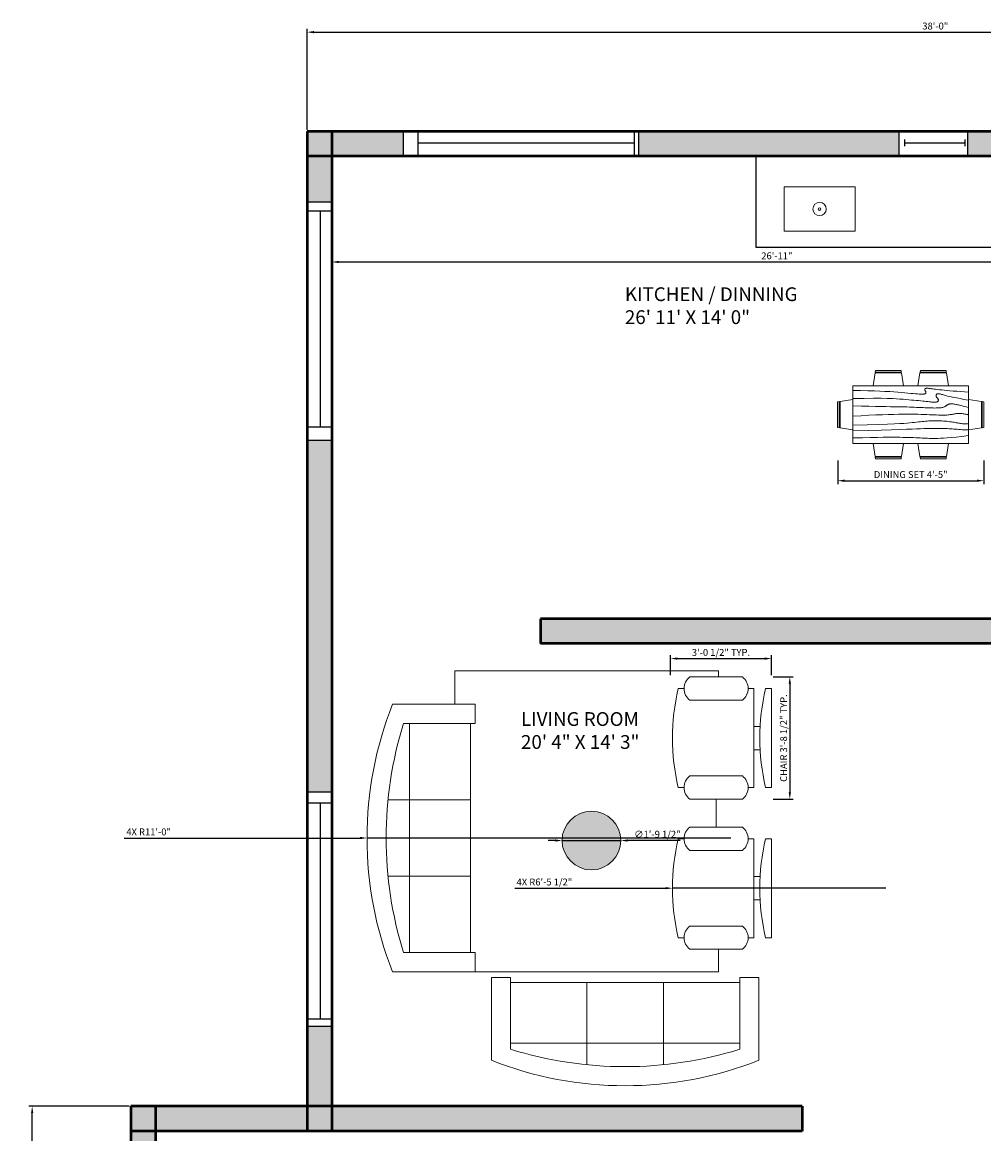
# Model space of a CAD drawing. Units: millimetres. Extents: x 2481 to 3088, y 720 to 1513.
# Tile 3 of 4: x 2487 to 2836, y 1109 to 1513. Entities that reach past the tile are written whole.
import ezdxf

# ---------------------------------------------------------------- set-up
doc = ezdxf.new("R2010")
doc.units = ezdxf.units.MM
for name, color, linetype, lineweight in [('A-FLOR-CASE', 150, 'Continuous', 25), ('A-FLOR-FIXT', 2, 'Continuous', 18), ('A-FURN-PATT', 3, 'Continuous', 13), ('A-WALL-PATT', 5, 'Continuous', 13), ('DIMENSIONS', 10, 'Continuous', 18), ('FURNITURE', 2, 'Continuous', 18), ('TEXT', 80, 'Continuous', 25), ('WALLS', 150, 'Continuous', 50), ('WINDOWS', 23, 'Continuous', 25)]:
    doc.layers.add(name, color=color, linetype=linetype, lineweight=lineweight)
doc.styles.get("Standard").update_dxf_attribs({"font": 'arial.ttf'})
doc.dimstyles.new('ISO-25', dxfattribs={"dimtxt": 2.5, "dimasz": 2.5, "dimexe": 1.25, "dimexo": 0.625, "dimtad": 1, "dimdec": 0, "dimlunit": 3, "dimtxsty": 'Standard', "dimcen": 2.5, "dimadec": 0, "dimazin": 0, "dimtfac": 1, "dimtdec": 0, "dimtmove": 0, "dimatfit": 3, "dimfxl": 1, "dimarcsym": 0})

# ---------------------------------------------------------------- blocks, each defined once
blk = doc.blocks.new('*U4')
for p, q in [((0, 4), (0, 0)), ((36, 4), (36, 0)), ((0, 2), (36, 2))]:
    blk.add_line(p, q)
blk = doc.blocks.new('*U6')
for p, q in [((0, 4), (0, 0)), ((0, 2), (36, 2)), ((36, 4), (36, 0))]:
    blk.add_line(p, q)
blk = doc.blocks.new('Dining Set - 36 x 72 in.')
for p, q in [((-22.2343, 26.00059), (-23.4847, 17.99762)), ((-22.2304, 26), (-5.7608, 26)), ((-22, 27.5), (-22.1562, 26.50042)), ((-5.8416, 26.5), (-22.1534, 26.5)), ((-22, 27.5), (-6, 27.5)), ((-5.8437, 26.49966), (-6, 27.5)), ((-4.5152, 17.99762), (-5.7655, 25.99926)), ((5.7657, 26.00059), (4.5153, 17.99762)), ((5.7696, 26), (22.2392, 26)), ((6, 27.5), (5.8438, 26.50042)), ((22.1584, 26.5), (5.8466, 26.5)), ((6, 27.5), (22, 27.5)), ((22.1563, 26.49966), (22, 27.5)), ((23.4848, 17.99762), (22.2345, 25.99926)), ((36, 18), (-36, 18)), ((-36, 18), (-36, -18)), ((36, -18), (36, 18)), ((-45.5, 8), (-44.5004, 8.15617)), ((-45.5, 8), (-45.5, -8)), ((-44.5, -8.15843), (-44.5, 8.15338)), ((-44.0006, 8.23428), (-35.9976, 9.48474)), ((-44, 8.23041), (-44, -8.23915)), ((44.0006, 8.23428), (35.9976, 9.48474)), ((44, 8.23041), (44, -8.23915)), ((44.5, -8.15843), (44.5, 8.15338)), ((45.5, 8), (44.5005, 8.15617)), ((45.5, 8), (45.5, -8)), ((-44.4997, -8.15631), (-45.5, -8)), ((-35.9976, -9.48476), (-43.9993, -8.2345)), ((35.9976, -9.48476), (43.9993, -8.2345)), ((44.4997, -8.15631), (45.5, -8)), ((-36, -18), (36, -18)), ((-22.2343, -26.0006), (-23.4847, -17.99762)), ((-4.5152, -17.99762), (-5.7655, -25.99928)), ((5.7657, -26.0006), (4.5153, -17.99762)), ((23.4848, -17.99762), (22.2345, -25.99928)), ((-22.2304, -26), (-5.7608, -26)), ((-22, -27.5), (-22.1562, -26.50044)), ((-5.8416, -26.5), (-22.1534, -26.5)), ((-22, -27.5), (-6, -27.5)), ((-5.8437, -26.49967), (-6, -27.5)), ((5.7696, -26), (22.2392, -26)), ((6, -27.5), (5.8438, -26.50044)), ((22.1584, -26.5), (5.8466, -26.5)), ((6, -27.5), (22, -27.5)), ((22.1563, -26.49967), (22, -27.5))]:
    blk.add_line(p, q)
for points in [[(-36, 15), (-31.1772, 14.97754), (-26.8079, 14.91406), (-22.8538, 14.81543), (-19.276, 14.6875), (-16.0362, 14.53613), (-13.0957, 14.36718), (-10.4159, 14.18652), (-7.9583, 14), (-5.6904, 13.81315), (-3.6035, 13.63021), (-1.6954, 13.45508), (0.0365, 13.29166), (1.5945, 13.14388), (2.9811, 13.01562), (4.1988, 12.9108), (5.25, 12.83333), (6.1393, 12.78613), (6.8802, 12.76823), (7.4883, 12.77767), (7.9792, 12.8125), (8.3685, 12.87077), (8.6719, 12.95052), (8.9049, 13.0498), (9.0833, 13.16666), (9.2205, 13.29899), (9.3216, 13.44401), (9.3895, 13.59879), (9.4271, 13.76041), (9.4373, 13.92594), (9.4232, 14.09245), (9.3875, 14.257), (9.3333, 14.41666), (9.2638, 14.56917), (9.1836, 14.71484), (9.0975, 14.85465), (9.0104, 14.98958), (8.9272, 15.1206), (8.8529, 15.2487), (8.7922, 15.37483), (8.75, 15.5), (8.7305, 15.62467), (8.7344, 15.74739), (8.7617, 15.86621), (8.8125, 15.97916), (8.8867, 16.08431), (8.9844, 16.17968), (9.1055, 16.26334), (9.25, 16.33333), (9.4189, 16.38802), (9.6172, 16.42708), (9.8506, 16.45052), (10.125, 16.45833), (10.4463, 16.45052), (10.8203, 16.42708), (11.2529, 16.38802), (11.75, 16.33333), (12.3184, 16.26318), (12.9694, 16.17838), (13.7151, 16.07991), (14.5677, 15.96875), (15.5395, 15.84586), (16.6426, 15.71224), (17.8893, 15.56884), (19.2917, 15.41666), (20.859, 15.25667), (22.5879, 15.08984), (24.4721, 14.91715), (26.5052, 14.73958), (28.6809, 14.5581), (30.9929, 14.3737), (33.4347, 14.18733), (36, 14)], [(-36, 10), (-28.9766, 10.14274), (-23.1725, 10.20442), (-18.4241, 10.19775), (-14.5677, 10.13541), (-11.4399, 10.03011), (-8.877, 9.89453), (-6.7154, 9.74137), (-4.7917, 9.58333), (-2.9698, 9.43082), (-1.2246, 9.28515), (0.4415, 9.14534), (2.026, 9.01041), (3.5266, 8.87939), (4.9408, 8.7513), (6.266, 8.62516), (7.5, 8.5), (8.6411, 8.37549), (9.6914, 8.2539), (10.6538, 8.13818), (11.5312, 8.03125), (12.3267, 7.93603), (13.043, 7.85547), (13.6831, 7.79248), (14.25, 7.75), (14.7471, 7.7303), (15.1797, 7.73307), (15.5537, 7.75732), (15.875, 7.80208), (16.1494, 7.86637), (16.3828, 7.94922), (16.5811, 8.04964), (16.75, 8.16666), (16.8944, 8.29915), (17.0143, 8.44531), (17.1089, 8.60319), (17.1771, 8.77083), (17.218, 8.94629), (17.2305, 9.1276), (17.2137, 9.31282), (17.1667, 9.5), (17.0895, 9.6875), (16.987, 9.875), (16.8649, 10.0625), (16.7292, 10.25), (16.5856, 10.4375), (16.4401, 10.625), (16.2985, 10.8125), (16.1667, 11), (16.05, 11.18733), (15.9518, 11.3737), (15.8752, 11.5581), (15.8229, 11.73958), (15.798, 11.91715), (15.8034, 12.08984), (15.842, 12.25667), (15.9167, 12.41666), (16.0295, 12.56836), (16.1784, 12.70833), (16.3605, 12.83268), (16.5729, 12.9375), (16.8127, 13.01888), (17.0768, 13.07291), (17.3625, 13.0957), (17.6667, 13.08333), (17.9894, 13.03312), (18.3418, 12.94726), (18.7382, 12.82918), (19.1927, 12.68229), (19.7195, 12.51001), (20.3327, 12.31575), (21.0465, 12.10294), (21.875, 11.875), (22.8357, 11.63354), (23.959, 11.37304), (25.2786, 11.08618), (26.8282, 10.76562), (28.6414, 10.40405), (30.752, 9.99414), (33.1936, 9.52856), (36, 9)], [(-36, 5.5), (-30.7157, 5.3348), (-26.069, 5.20963), (-21.9946, 5.11767), (-18.4271, 5.05208), (-15.3009, 5.00602), (-12.5508, 4.97265), (-10.1112, 4.94515), (-7.9167, 4.91666), (-5.909, 4.88167), (-4.0586, 4.83984), (-2.3429, 4.79215), (-0.7396, 4.73958), (0.7739, 4.6831), (2.22, 4.6237), (3.6213, 4.56233), (5, 4.5), (6.373, 4.43782), (7.7344, 4.3776), (9.0723, 4.32129), (10.375, 4.27083), (11.6309, 4.22819), (12.8281, 4.19531), (13.9551, 4.17415), (15, 4.16666), (15.954, 4.17448), (16.819, 4.19791), (17.6001, 4.23698), (18.3021, 4.29166), (18.9299, 4.36198), (19.4883, 4.44791), (19.9823, 4.54948), (20.4167, 4.66666), (20.7969, 4.79899), (21.1302, 4.94401), (21.4245, 5.09879), (21.6875, 5.26041), (21.9271, 5.42594), (22.1511, 5.59245), (22.3672, 5.757), (22.5834, 5.91666), (22.8065, 6.06868), (23.0404, 6.21093), (23.2879, 6.34147), (23.5521, 6.45833), (23.8358, 6.55957), (24.142, 6.64323), (24.4735, 6.70735), (24.8334, 6.75), (25.2235, 6.76969), (25.642, 6.76692), (26.0858, 6.74267), (26.5521, 6.69791), (27.0379, 6.63362), (27.5404, 6.55078), (28.0565, 6.45036), (28.5834, 6.33333), (29.1242, 6.19987), (29.7071, 6.04687), (30.3661, 5.87044), (31.1354, 5.66666), (32.0493, 5.43164), (33.142, 5.16146), (34.4475, 4.85221), (36, 4.5)], [(-36, -1), (-30.7915, -0.6591), (-26.0195, -0.38216), (-21.6519, -0.16284), (-17.6563, 0.00521), (-14.0005, 0.12833), (-10.6523, 0.21289), (-7.5796, 0.26522), (-4.75, 0.29166), (-2.134, 0.29793), (0.2878, 0.28711), (2.5317, 0.26163), (4.6146, 0.22396), (6.5529, 0.17651), (8.3633, 0.12174), (10.0623, 0.06209), (11.6667, 0), (13.1899, -0.06201), (14.6341, -0.1211), (15.9982, -0.17432), (17.2813, -0.21875), (18.4823, -0.25147), (19.6003, -0.26953), (20.6343, -0.27002), (21.5834, -0.25), (22.4481, -0.20768), (23.2357, -0.14584), (23.9549, -0.06836), (24.6146, 0.02083), (25.2235, 0.11784), (25.7904, 0.21875), (26.3241, 0.31966), (26.8334, 0.41666), (27.3265, 0.50618), (27.8099, 0.58593), (28.2894, 0.65397), (28.7709, 0.70833), (29.2601, 0.74707), (29.763, 0.76823), (30.2855, 0.76985), (30.8334, 0.75), (31.4088, 0.70784), (31.9994, 0.64713), (32.589, 0.57275), (33.1615, 0.48958), (33.7008, 0.4025), (34.1908, 0.3164), (34.6153, 0.23616), (34.9584, 0.16666), (35.2099, 0.11165), (35.3848, 0.07031), (35.504, 0.04069), (35.5886, 0.02083), (35.6594, 0.00879), (35.7377, 0.0026), (35.8442, 0.00032), (36, 0)], [(-36, -6.5), (-27.1843, -6.31267), (-20.084, -6.1263), (-14.469, -5.9419), (-10.1094, -5.76042), (-6.7752, -5.58285), (-4.2363, -5.41016), (-2.2629, -5.24333), (-0.625, -5.08334), (0.8708, -4.93099), (2.2715, -4.78646), (3.5872, -4.64974), (4.8281, -4.52084), (6.0046, -4.39974), (7.127, -4.28646), (8.2053, -4.18099), (9.25, -4.08334), (10.2705, -3.99382), (11.2734, -3.91407), (12.2647, -3.84603), (13.25, -3.79167), (14.2354, -3.75293), (15.2266, -3.73177), (16.2295, -3.73015), (17.25, -3.75), (18.2912, -3.79248), (19.3451, -3.85547), (20.4009, -3.93604), (21.4479, -4.03125), (22.4754, -4.13819), (23.4727, -4.25391), (24.4289, -4.37549), (25.3334, -4.5), (26.1785, -4.62492), (26.9694, -4.74935), (27.7145, -4.87281), (28.4219, -4.99479), (29.1, -5.11483), (29.7572, -5.23242), (30.4016, -5.34709), (31.0417, -5.45834), (31.6837, -5.56437), (32.3262, -5.65821), (32.9658, -5.73153), (33.599, -5.77604), (34.2224, -5.78345), (34.8327, -5.74545), (35.4264, -5.65373), (36, -5.5)], [(-36, -10), (-26.4022, -9.81299), (-18.4675, -9.62891), (-11.9839, -9.45069), (-6.7396, -9.28125), (-2.5226, -9.12354), (0.8789, -8.98047), (3.6769, -8.85498), (6.0833, -8.75), (8.2767, -8.66765), (10.3021, -8.60677), (12.1712, -8.56543), (13.8958, -8.54167), (15.4876, -8.53353), (16.9583, -8.53907), (18.3197, -8.55632), (19.5834, -8.58334), (20.7616, -8.61841), (21.8685, -8.66081), (22.9188, -8.71004), (23.9271, -8.76563), (24.9081, -8.82707), (25.8763, -8.89388), (26.8465, -8.96558), (27.8334, -9.04167), (28.8474, -9.12118), (29.8828, -9.20117), (30.93, -9.27824), (31.9792, -9.34896), (33.0205, -9.40991), (34.0443, -9.45768), (35.0407, -9.48885), (36, -9.5)], [(-36, -14.5), (-30.0881, -14.33513), (-25.0332, -14.21224), (-20.7312, -14.12647), (-17.0781, -14.07292), (-13.97, -14.04671), (-11.3027, -14.04297), (-8.9724, -14.05681), (-6.875, -14.08334), (-4.9224, -14.11833), (-3.0905, -14.16016), (-1.3709, -14.20785), (0.2448, -14.26042), (1.7647, -14.3169), (3.1973, -14.3763), (4.5507, -14.43767), (5.8333, -14.5), (7.0554, -14.5621), (8.235, -14.62175), (9.3922, -14.67652), (10.5469, -14.72396), (11.7192, -14.76164), (12.929, -14.78711), (14.1965, -14.79794), (15.5417, -14.79167), (16.9933, -14.76424), (18.6152, -14.70508), (20.4804, -14.60197), (22.6615, -14.44271), (25.2312, -14.21509), (28.2624, -13.9069), (31.8277, -13.50594), (36, -13)]]:
    blk.add_lwpolyline(points)
blk = doc.blocks.new('Sofa - Roundback 7 ft.')
for p, q in [((-12.00002, -32.4421), (-12.00003, -6.5971)), ((11.99997, -32.4421), (11.99998, -6.5971)), ((-36.000027, -34), (-36.000027, -11.4696)), ((-35.999844, -13.3819), (35.9998, -13.3819)), ((35.99998, -34), (35.99998, -11.4696)), ((-36.000027, -32.4421), (35.99998, -32.4421))]:
    blk.add_line(p, q)
for points in [[(-36.000027, -34), (-42.000027, -34), (-42.000027, -8)], [(41.99998, -8), (41.99998, -34), (35.99998, -34)]]:
    blk.add_lwpolyline(points)
for centre, radius, start, end in [((0, -114.25), 114.25, 68.43141, 111.5686), ((-0.00001, -127.1968), 121.1968, 72.72033, 107.2797)]:
    blk.add_arc(centre, radius, start, end)
blk = doc.blocks.new('Chair - Desk')
for p, q in [((-8.5, 0), (-8.5, -1)), ((-8.5, 0), (8.5, 0)), ((8.5, 0), (8.5, -1)), ((-8.5, -3), (-8.5, -4)), ((-8.5, -3), (8.5, -3)), ((-2, -3), (-2, -1.9355)), ((2, -1.9576), (2, -3)), ((8.5, -3), (8.5, -4)), ((-10.5, -5), (-10.5, -14)), ((-6.5, -14), (-6.5, -5)), ((6.5, -5), (6.5, -14)), ((10.5, -14), (10.5, -5)), ((-8.5, -15), (-8.5, -16)), ((8.5, -15), (8.5, -16))]:
    blk.add_line(p, q)
for centre, radius, start, end in [((0, 34.625), 36.625, 256.5803, 283.4197), ((-8.5, -6.5), 2.5, 36.8699, 143.1301), ((8.5, -6.5), 2.5, 36.8699, 143.1301), ((-8.5, -12.5), 2.5, 216.8699, 323.1301), ((8.5, -12.5), 2.5, 216.8699, 323.1301), ((0, 19.625), 36.625, 256.5803, 283.4197)]:
    blk.add_arc(centre, radius, start, end)
blk = doc.blocks.new('*D16')
at = {"layer": 'Defpoints', "color": 0, "transparency": 16777216}
for p in [(2599.5, 1428.42), (2922.5, 1426.09), (2922.5, 1426.09)]:
    blk.add_point(p, dxfattribs=at)
at = {"layer": 'DIMENSIONS', "color": 0, "lineweight": -2, "transparency": 16777216}
for p, q in [((2599.5, 1427.79), (2599.5, 1424.84)), ((2602, 1426.09), (2920, 1426.09)), ((2922.5, 1426.72), (2922.5, 1427.34))]:
    blk.add_line(p, q, dxfattribs=at)
at = {"layer": 'DIMENSIONS', "color": 0, "transparency": 16777216}
for points in [[(2602, 1426.51), (2602, 1425.68), (2599.5, 1426.09)], [(2920, 1426.51), (2920, 1425.68), (2922.5, 1426.09)]]:
    blk.add_solid(points, dxfattribs=at)
at = {"layer": 'DIMENSIONS', "color": 0, "transparency": 16777216, "insert": (2761, 1428), "char_height": 2.5, "attachment_point": 5}
blk.add_mtext('26\'-11"', dxfattribs=at)
blk = doc.blocks.new('*D29')
at = {"layer": 'Defpoints', "color": 0, "transparency": 16777216}
for p in [(2759.04, 1275.4), (2759.04, 1230.99), (2765.7, 1230.99)]:
    blk.add_point(p, dxfattribs=at)
at = {"layer": 'DIMENSIONS', "color": 0, "lineweight": -2, "transparency": 16777216}
for p, q in [((2759.66, 1275.4), (2766.95, 1275.4)), ((2765.7, 1272.9), (2765.7, 1233.49)), ((2759.66, 1230.99), (2766.95, 1230.99))]:
    blk.add_line(p, q, dxfattribs=at)
at = {"layer": 'DIMENSIONS', "color": 0, "transparency": 16777216}
for points in [[(2765.28, 1272.9), (2766.11, 1272.9), (2765.7, 1275.4)], [(2765.28, 1233.49), (2766.11, 1233.49), (2765.7, 1230.99)]]:
    blk.add_solid(points, dxfattribs=at)
at = {"layer": 'DIMENSIONS', "color": 0, "transparency": 16777216, "insert": (2763.78, 1253.19), "char_height": 2.5, "attachment_point": 5, "rotation": 90}
blk.add_mtext('CHAIR 3\'-8 1/2" TYP.', dxfattribs=at)
blk = doc.blocks.new('*D30')
at = {"layer": 'Defpoints', "color": 0, "transparency": 16777216}
for p in [(2759.04, 1282.06), (2722.39, 1275.4), (2759.04, 1275.4)]:
    blk.add_point(p, dxfattribs=at)
at = {"layer": 'DIMENSIONS', "color": 0, "lineweight": -2, "transparency": 16777216}
for p, q in [((2722.39, 1276.02), (2722.39, 1283.31)), ((2724.89, 1282.06), (2756.54, 1282.06)), ((2759.04, 1276.02), (2759.04, 1283.31))]:
    blk.add_line(p, q, dxfattribs=at)
at = {"layer": 'DIMENSIONS', "color": 0, "transparency": 16777216}
for points in [[(2724.89, 1282.47), (2724.89, 1281.64), (2722.39, 1282.06)], [(2756.54, 1282.47), (2756.54, 1281.64), (2759.04, 1282.06)]]:
    blk.add_solid(points, dxfattribs=at)
at = {"layer": 'DIMENSIONS', "color": 0, "transparency": 16777216, "insert": (2740.71, 1283.97), "char_height": 2.5, "attachment_point": 5}
blk.add_mtext('3\'-0 1/2" TYP.', dxfattribs=at)
blk = doc.blocks.new('*D33')
at = {"layer": 'Defpoints', "color": 0, "transparency": 16777216}
for p in [(2783.07, 1354.61), (2836.1, 1354.61), (2836.1, 1346.66)]:
    blk.add_point(p, dxfattribs=at)
at = {"layer": 'DIMENSIONS', "color": 0, "lineweight": -2, "transparency": 16777216}
for p, q in [((2783.07, 1353.98), (2783.07, 1345.41)), ((2836.1, 1353.98), (2836.1, 1345.41)), ((2785.57, 1346.66), (2833.6, 1346.66))]:
    blk.add_line(p, q, dxfattribs=at)
at = {"layer": 'DIMENSIONS', "color": 0, "transparency": 16777216}
for points in [[(2785.57, 1347.07), (2785.57, 1346.24), (2783.07, 1346.66)], [(2833.6, 1347.07), (2833.6, 1346.24), (2836.1, 1346.66)]]:
    blk.add_solid(points, dxfattribs=at)
at = {"layer": 'DIMENSIONS', "color": 0, "transparency": 16777216, "insert": (2809.58, 1348.57), "char_height": 2.5, "attachment_point": 5}
blk.add_mtext('DINING SET 4\'-5"', dxfattribs=at)
blk = doc.blocks.new('*D39')
at = {"layer": 'Defpoints', "color": 0, "transparency": 16777216}
for p in [(3046.5, 1509.55), (2590.5, 1473.49), (3046.5, 1473.49)]:
    blk.add_point(p, dxfattribs=at)
at = {"layer": 'DIMENSIONS', "color": 0, "lineweight": -2, "transparency": 16777216}
for p, q in [((2590.5, 1474.11), (2590.5, 1510.8)), ((3046.5, 1474.11), (3046.5, 1510.8)), ((2593, 1509.55), (3044, 1509.55))]:
    blk.add_line(p, q, dxfattribs=at)
at = {"layer": 'DIMENSIONS', "color": 0, "transparency": 16777216}
for points in [[(2593, 1509.97), (2593, 1509.13), (2590.5, 1509.55)], [(3044, 1509.97), (3044, 1509.13), (3046.5, 1509.55)]]:
    blk.add_solid(points, dxfattribs=at)
at = {"layer": 'DIMENSIONS', "color": 0, "transparency": 16777216, "insert": (2818.5, 1511.45), "char_height": 2.5, "attachment_point": 5}
blk.add_mtext('38\'-0"', dxfattribs=at)
blk = doc.blocks.new('*D40')
at = {"layer": 'Defpoints', "color": 0, "transparency": 16777216}
for p in [(2490.69, 1119.49), (2526.5, 1119.49), (2526.5, 765.49)]:
    blk.add_point(p, dxfattribs=at)
at = {"layer": 'DIMENSIONS', "color": 0, "lineweight": -2, "transparency": 16777216}
for p, q in [((2525.87, 1119.49), (2489.44, 1119.49)), ((2490.69, 767.99), (2490.69, 1116.99)), ((2525.87, 765.49), (2489.44, 765.49))]:
    blk.add_line(p, q, dxfattribs=at)
at = {"layer": 'DIMENSIONS', "color": 0, "transparency": 16777216}
for points in [[(2490.28, 1116.99), (2491.11, 1116.99), (2490.69, 1119.49)], [(2490.28, 767.99), (2491.11, 767.99), (2490.69, 765.49)]]:
    blk.add_solid(points, dxfattribs=at)
at = {"layer": 'DIMENSIONS', "color": 0, "transparency": 16777216, "insert": (2488.79, 942.49), "char_height": 2.5, "attachment_point": 5, "rotation": 90}
blk.add_mtext('29\'-6"', dxfattribs=at)
blk = doc.blocks.new('*D48')
at = {"layer": 'Defpoints', "color": 0, "transparency": 16777216}
for p in [(2612.23, 1216.89), (2744.32, 1216.89)]:
    blk.add_point(p, dxfattribs=at)
at = {"layer": 'DIMENSIONS', "color": 0, "lineweight": -2, "transparency": 16777216}
for p, q in [((2524.12, 1216.89), (2609.73, 1216.89)), ((2744.32, 1216.89), (2612.23, 1216.89))]:
    blk.add_line(p, q, dxfattribs=at)
at = {"layer": 'DIMENSIONS', "color": 0, "transparency": 16777216}
blk.add_solid([(2609.73, 1217.31), (2609.73, 1216.48), (2612.23, 1216.89)], dxfattribs=at)
at = {"layer": 'DIMENSIONS', "color": 0, "transparency": 16777216, "insert": (2532.97, 1218.79), "char_height": 2.5, "attachment_point": 5, "rotation": 359.9998}
blk.add_mtext('4X R11\'-0"', dxfattribs=at)
blk = doc.blocks.new('*D49')
at = {"layer": 'Defpoints', "color": 0, "transparency": 16777216}
for p in [(2723.09, 1198.67), (2800.53, 1198.67)]:
    blk.add_point(p, dxfattribs=at)
at = {"layer": 'DIMENSIONS', "color": 0, "lineweight": -2, "transparency": 16777216}
for p, q in [((2665.84, 1198.67), (2720.59, 1198.67)), ((2800.53, 1198.67), (2723.09, 1198.67))]:
    blk.add_line(p, q, dxfattribs=at)
at = {"layer": 'DIMENSIONS', "color": 0, "transparency": 16777216}
blk.add_solid([(2720.59, 1199.09), (2720.59, 1198.26), (2723.09, 1198.67)], dxfattribs=at)
at = {"layer": 'DIMENSIONS', "color": 0, "transparency": 16777216, "insert": (2676.63, 1200.59), "char_height": 2.5, "attachment_point": 5, "rotation": 359.9998}
blk.add_mtext('4X R6\'-5 1/2"', dxfattribs=at)
blk = doc.blocks.new('*D52')
at = {"layer": 'Defpoints', "color": 0, "transparency": 16777216}
for p in [(2683.03, 1215.98), (2704.4, 1215.98)]:
    blk.add_point(p, dxfattribs=at)
at = {"layer": 'DIMENSIONS', "color": 0, "lineweight": -2, "transparency": 16777216}
for p, q in [((2680.53, 1215.98), (2678.03, 1215.98)), ((2683.03, 1215.98), (2704.4, 1215.98)), ((2725.84, 1215.98), (2706.9, 1215.98))]:
    blk.add_line(p, q, dxfattribs=at)
at = {"layer": 'DIMENSIONS', "color": 0, "transparency": 16777216}
for points in [[(2680.53, 1216.4), (2680.53, 1215.56), (2683.03, 1215.98)], [(2706.9, 1216.4), (2706.9, 1215.56), (2704.4, 1215.98)]]:
    blk.add_solid(points, dxfattribs=at)
at = {"layer": 'DIMENSIONS', "color": 0, "transparency": 16777216, "insert": (2717.62, 1217.95), "char_height": 2.5, "attachment_point": 5, "rotation": 0.0003}
blk.add_mtext('∅1\'-9 1/2"', dxfattribs=at)

msp = doc.modelspace()

# ---------------------------------------------------------------- hatches: boundary and pattern name
at = {"layer": 'A-FURN-PATT'}
h = msp.add_hatch(color=256, dxfattribs=at)
h.dxf.hatch_style = 1
h.paths.add_polyline_path([(2704.4, 1215.98, 1), (2683.03, 1215.98, 1)])
at = {"layer": 'A-WALL-PATT'}
h = msp.add_hatch(color=256, dxfattribs=at)
h.dxf.hatch_style = 1
h.paths.add_polyline_path([(2599.5, 1473.49), (2590.5, 1473.49), (2590.5, 1464.49), (2599.5, 1464.49)])
h.paths.add_polyline_path([(2599.5, 1464.49), (2590.5, 1464.49), (2590.5, 1447.8), (2599.5, 1447.8)])
h.paths.add_polyline_path([(2625.38, 1473.49), (2599.5, 1473.49), (2599.5, 1464.49), (2625.38, 1464.49)])
h.paths.add_polyline_path([(2805.36, 1473.49), (2710.95, 1473.49), (2710.95, 1464.49), (2805.36, 1464.49)])
h.paths.add_polyline_path([(2922.5, 1473.49), (2830.18, 1473.49), (2830.18, 1464.49), (2922.5, 1464.49)])
h.paths.add_polyline_path([(2931.5, 1473.49), (2922.5, 1473.49), (2922.5, 1464.49), (2931.5, 1464.49)])
h.paths.add_polyline_path([(2931.5, 1464.49), (2922.5, 1464.49), (2922.5, 1402.56), (2926.01, 1402.56, -0.043673), (2931.5, 1402.08)])
h.paths.add_polyline_path([(2931.5, 1368.49), (2922.5, 1368.49), (2922.5, 1359.49), (2931.5, 1359.49)])
h.paths.add_polyline_path([(2922.5, 1296.49), (2675.15, 1296.49), (2675.15, 1287.49), (2922.5, 1287.49)])
h.paths.add_polyline_path([(2931.5, 1294.49), (2922.5, 1294.49), (2922.5, 1287.49), (2922.5, 1285.49), (2931.5, 1285.49)])
h.paths.add_polyline_path([(3037.5, 1294.49), (2931.5, 1294.49), (2931.5, 1285.49), (3037.5, 1285.49)])
h.paths.add_polyline_path([(3046.5, 1294.49), (3037.5, 1294.49), (3037.5, 1285.49), (3046.5, 1285.49)])
h.paths.add_polyline_path([(3046.5, 1316.66), (3037.5, 1316.66), (3037.5, 1294.49), (3046.5, 1294.49)])
h.paths.add_polyline_path([(3046.5, 1359.49), (3037.5, 1359.49), (3037.5, 1343.26), (3046.5, 1343.26)])
h.paths.add_polyline_path([(3046.5, 1368.49), (3037.5, 1368.49), (3037.5, 1359.49), (3046.5, 1359.49)])
h.paths.add_polyline_path([(3037.5, 1368.49), (2931.5, 1368.49), (2931.5, 1359.49), (3037.5, 1359.49)])
h.paths.add_polyline_path([(2599.5, 1361.25), (2590.5, 1361.25), (2590.5, 1233.6), (2599.5, 1233.6)])
h.paths.add_polyline_path([(2535.5, 1110.49), (2526.5, 1110.49), (2526.5, 933.49), (2535.5, 933.49)])
h.paths.add_polyline_path([(2535.5, 1119.49), (2526.5, 1119.49), (2526.5, 1110.49), (2535.5, 1110.49)])
h.paths.add_polyline_path([(2590.5, 1119.49), (2535.5, 1119.49), (2535.5, 1110.49), (2590.5, 1110.49)])
h.paths.add_polyline_path([(2599.5, 1119.49), (2594.5, 1119.49), (2590.5, 1119.49), (2590.5, 1110.49), (2594.5, 1110.49), (2599.5, 1110.49)])
h.paths.add_polyline_path([(2599.5, 1148.41), (2590.5, 1148.41), (2590.5, 1119.49), (2594.5, 1119.49), (2599.5, 1119.49)])
h.paths.add_polyline_path([(2770.14, 1119.49), (2599.5, 1119.49), (2599.5, 1110.49), (2770.14, 1110.49)])
h.paths.add_polyline_path([(3037.5, 1473.49), (2931.5, 1473.49), (2931.5, 1464.49), (3037.5, 1464.49)])
h.paths.add_polyline_path([(3046.5, 1473.49), (3037.5, 1473.49), (3037.5, 1464.49), (3046.5, 1464.49)])
h.paths.add_polyline_path([(2535.5, 842.83), (2535.5, 924.49), (2526.5, 924.49), (2526.5, 774.49), (2535.5, 774.49)])
h.paths.add_polyline_path([(2535.5, 774.49), (2526.5, 774.49), (2526.5, 765.49), (2535.5, 765.49)])
h.paths.add_polyline_path([(3037.5, 774.49), (2945.5, 774.49), (2852.34, 774.49), (2852.34, 765.49), (3037.5, 765.49)])
h.paths.add_polyline_path([(3046.5, 774.49), (3037.5, 774.49), (3037.5, 765.49), (3046.5, 765.49)])
h.paths.add_polyline_path([(3046.5, 882.49), (3037.5, 882.49), (3037.5, 774.49), (3046.5, 774.49)])
h.paths.add_polyline_path([(2768.5, 774.49), (2759.5, 774.49), (2759.5, 765.49), (2768.5, 765.49)])
h.paths.add_polyline_path([(2759.5, 774.49), (2535.5, 774.49), (2535.5, 765.49), (2759.5, 765.49)])
h.paths.add_polyline_path([(2768.5, 781.94), (2759.5, 781.94), (2759.5, 774.49), (2768.5, 774.49)])
h.paths.add_polyline_path([(2768.5, 1015.49), (2759.5, 1015.49), (2759.5, 933.49), (2768.5, 933.49)])
h.paths.add_polyline_path([(2768.5, 933.49), (2759.5, 933.49), (2759.5, 924.49), (2768.5, 924.49)])
h.paths.add_polyline_path([(2768.5, 924.49), (2759.5, 924.49), (2759.5, 864.16), (2768.5, 864.16)])
h.paths.add_polyline_path([(2759.5, 933.49), (2734.57, 933.49), (2734.57, 924.49), (2759.5, 924.49)])
h.paths.add_polyline_path([(2954.5, 1015.49), (2945.5, 1015.49), (2945.5, 842.83), (2954.5, 842.83)])
h.paths.add_polyline_path([(2954.5, 1024.49), (2945.5, 1024.49), (2945.5, 1015.49), (2954.5, 1015.49)])
h.paths.add_polyline_path([(2945.5, 1024.49), (2808.62, 1024.49), (2808.62, 1022.52, -0.056199), (2807.82, 1015.49), (2945.5, 1015.49)])
h.paths.add_polyline_path([(3037.5, 1024.49), (2954.5, 1024.49), (2954.5, 1015.49), (3037.5, 1015.49)])
h.paths.add_polyline_path([(3046.5, 1024.49), (3037.5, 1024.49), (3037.5, 1015.49), (3046.5, 1015.49)])
h.paths.add_polyline_path([(3046.5, 1015.49), (3037.5, 1015.49), (3037.5, 994.13), (3046.5, 994.13)])
h.paths.add_polyline_path([(3046.5, 928.1), (3037.5, 928.1), (3037.5, 891.49), (3046.5, 891.49)])
h.paths.add_polyline_path([(3046.5, 891.49), (3037.5, 891.49), (3037.5, 882.49), (3046.5, 882.49)])
h.paths.add_polyline_path([(3037.5, 891.49), (2987.62, 891.49), (2987.62, 882.49), (3037.5, 882.49)])
h.paths.add_polyline_path([(2768.5, 1024.49), (2759.5, 1024.49), (2759.5, 1015.49), (2768.5, 1015.49)])
h.paths.add_polyline_path([(2777.03, 1022.52), (2777.03, 1024.49), (2768.5, 1024.49), (2768.5, 1015.49), (2777.03, 1015.49)])

# ---------------------------------------------------------------- linework, layer by layer
at = {"layer": 'A-FLOR-CASE'}
for p, q in [((2753.35, 1464.49), (2753.35, 1431.44)), ((2753.35, 1431.44), (2922.5, 1431.44))]:
    msp.add_line(p, q, dxfattribs=at)
at = {"layer": 'A-FLOR-FIXT'}
msp.add_lwpolyline([(2763.64, 1453.4), (2789.37, 1453.4), (2789.37, 1437.23), (2763.64, 1437.23)], close=True, dxfattribs=at)
for radius in [2.41, 2.41, 2.41, 0.486]:
    msp.add_circle((2776.51, 1445.32), radius, dxfattribs=at)
at = {"layer": 'FURNITURE'}
for p, q in [((2644.1, 1277.63), (2739.83, 1277.63)), ((2644.1, 1265.45), (2644.1, 1277.63)), ((2739.83, 1277.63), (2739.83, 1275.4)), ((2739.83, 1275.4), (2739.83, 1275.51)), ((2644.1, 1265.45), (2644.1, 1266.12)), ((2738.95, 1220.87), (2738.95, 1230.99)), ((2739.83, 1176.47), (2739.83, 1168.26)), ((2644.1, 1168.26), (2644.1, 1168.33)), ((2739.83, 1168.26), (2644.1, 1168.26))]:
    msp.add_line(p, q, dxfattribs=at)
msp.add_circle((2693.71, 1215.98), 10.68, dxfattribs=at)
at = {"layer": 'WALLS'}
for p, q in [((3046.5, 1473.49), (2590.5, 1473.49)), ((2590.5, 1473.49), (2590.5, 1110.49)), ((2599.5, 1473.49), (2599.5, 1110.49)), ((3046.5, 1464.49), (2590.5, 1464.49)), ((2922.5, 1296.49), (2675.15, 1296.49)), ((2675.15, 1296.49), (2675.15, 1287.49)), ((2922.5, 1287.49), (2675.15, 1287.49)), ((2590.5, 1119.49), (2526.5, 1119.49)), ((2526.5, 1119.49), (2526.5, 765.49)), ((2535.5, 1119.49), (2535.5, 774.49)), ((2594.5, 1119.49), (2590.5, 1119.49)), ((2770.14, 1119.49), (2594.5, 1119.49)), ((2770.14, 1119.49), (2770.14, 1110.49)), ((2590.5, 1110.49), (2526.5, 1110.49)), ((2594.5, 1110.49), (2590.5, 1110.49)), ((2770.14, 1110.49), (2594.5, 1110.49))]:
    msp.add_line(p, q, dxfattribs=at)
at = {"layer": 'WINDOWS'}
for p, q in [((2625.38, 1473.49), (2625.38, 1464.49)), ((2710.95, 1464.49), (2710.95, 1473.49)), ((2805.36, 1464.49), (2805.36, 1473.49)), ((2830.18, 1473.49), (2830.18, 1464.49)), ((2599.5, 1447.8), (2590.5, 1447.8)), ((2599.5, 1361.25), (2590.5, 1361.25)), ((2599.5, 1233.6), (2590.5, 1233.6)), ((2599.5, 1148.41), (2590.5, 1148.41))]:
    msp.add_line(p, q, dxfattribs=at)

# ---------------------------------------------------------------- block references
at = {"layer": 'FURNITURE', "xscale": 0.5827123837775617, "yscale": 0.5827123837775617, "zscale": 0.5827123837775617}
msp.add_blockref('Dining Set - 36 x 72 in.', (2809.58, 1370.63), dxfattribs=at)
at = {"layer": 'FURNITURE'}
for name, p, xscale, yscale, zscale, rotation in [('Chair - Desk', (2759.04, 1253.19), 2.114319489139201, 2.114319489139201, 2.114319489139201, 270), ('Sofa - Roundback 7 ft.', (2612.23, 1216.89), 1.15619311164389, 1.15619311164389, 1.15619311164389, 89.99999999999999), ('Chair - Desk', (2759.04, 1198.67), 2.114319489139201, 2.114319489139201, 2.114319489139201, 270), ('Sofa - Roundback 7 ft.', (2705.92, 1126.92), 1.15619311164389, 1.15619311164389, 1.15619311164389, 180)]:
    msp.add_blockref(name, p, dxfattribs=dict(at, xscale=xscale, yscale=yscale, zscale=zscale, rotation=rotation))
at = {"layer": 'WINDOWS'}
for name, p, xscale, yscale, zscale in [('*U4', (2630.71, 1465.03), 2.179725659021641, 2.179725659021641, 2.179725659021641), ('*U6', (2807.33, 1468.14), 0.6081270561735437, 0.6081270561735437, 0.6081270561735437)]:
    msp.add_blockref(name, p, dxfattribs=dict(at, xscale=xscale, yscale=yscale, zscale=zscale))
at = {"layer": 'WINDOWS', "xscale": 2.179725659021641, "yscale": 2.179725659021641, "zscale": 2.179725659021641, "rotation": 90}
for p in [(2599.71, 1366.21), (2599.71, 1151.26)]:
    msp.add_blockref('*U4', p, dxfattribs=at)

# ---------------------------------------------------------------- texts
at = {"layer": 'TEXT', "char_height": 5, "attachment_point": 1}
for s, width, insert in [('KITCHEN / DINNING \\P26\' 11\' X 14\' 0"', 86.8264, (2705.83, 1416.88)), ('LIVING ROOM \\P20\' 4" X 14\' 3"', 45.738, (2668.12, 1262.6))]:
    msp.add_mtext_dynamic_manual_height_columns(s, width=width, gutter_width=12.5, heights=[0], dxfattribs=dict(at, insert=insert))

# ---------------------------------------------------------------- dimensions: what is measured, and where the dimension line sits
at = {"layer": 'DIMENSIONS'}
for base, p1, p2, override, picture, middle in [((3046.5, 1509.55), (2590.5, 1473.49), (3046.5, 1473.49), {"dimdec": 1, "dimlfac": 1, "dimrnd": 0, "dimzin": 1, "dimdsep": 46, "dimlunit": 4, "dimfrac": 2}, '*D39', (2818.5, 1511.45)), ((2922.5, 1426.09), (2599.5, 1428.42), (2922.5, 1426.09), {"dimclrd": 0, "dimclre": 0, "dimclrt": 0}, '*D16', (2761, 1428))]:
    dim = msp.add_linear_dim(base=base, p1=p1, p2=p2, dimstyle='ISO-25', override=override, dxfattribs=at)
    dim.commit()
    dim.dimension.update_dxf_attribs({"geometry": picture, "text_midpoint": middle})
for base, p1, p2, text, picture, middle in [((2836.1, 1346.66), (2783.07, 1354.61), (2836.1, 1354.61), 'DINING SET <>', '*D33', (2809.58, 1348.57)), ((2759.0366, 1282.0551), (2722.3884, 1275.395), (2759.0366, 1275.395), '<> TYP.', '*D30', (2740.7125, 1283.9736))]:
    dim = msp.add_linear_dim(base=base, p1=p1, p2=p2, text=text, dimstyle='ISO-25', override={"dimdec": 1, "dimlfac": 1, "dimrnd": 0, "dimzin": 1, "dimdsep": 46, "dimlunit": 4, "dimfrac": 2}, dxfattribs=at)
    dim.commit()
    dim.dimension.update_dxf_attribs({"geometry": picture, "text_midpoint": middle})
dim = msp.add_linear_dim(base=(2765.7, 1230.99), p1=(2759.04, 1275.4), p2=(2759.04, 1230.99), angle=270, text='CHAIR <> TYP.', dimstyle='ISO-25', override={"dimdec": 1, "dimlfac": 1, "dimrnd": 0, "dimzin": 1, "dimdsep": 46, "dimlunit": 4, "dimfrac": 2}, dxfattribs=at)
dim.commit()
dim.dimension.update_dxf_attribs({"geometry": '*D29', "text_midpoint": (2763.78, 1253.19)})
for center, mpoint, picture, middle in [((2744.32, 1216.89), (2612.23, 1216.89), '*D48', (2532.97, 1216.89)), ((2800.53, 1198.67), (2723.09, 1198.67), '*D49', (2676.63, 1198.67))]:
    dim = msp.add_radius_dim(center=center, mpoint=mpoint, text='4X <>', dimstyle='ISO-25', override={"dimdec": 1, "dimlfac": 1, "dimrnd": 0, "dimzin": 1, "dimdsep": 46, "dimlunit": 4, "dimfrac": 2}, dxfattribs=at)
    dim.commit()
    dim.dimension.update_dxf_attribs({"geometry": picture, "text_midpoint": middle, "dimtype": 164})
dim = msp.add_diameter_dim_2p(p1=(2683.03, 1215.98), p2=(2704.4, 1215.98), dimstyle='ISO-25', override={"dimdec": 1, "dimlfac": 1, "dimrnd": 0, "dimzin": 1, "dimdsep": 46, "dimlunit": 4, "dimfrac": 2}, dxfattribs=at)
dim.commit()
dim.dimension.update_dxf_attribs({"geometry": '*D52', "text_midpoint": (2717.62, 1215.98)})
dim = msp.add_linear_dim(base=(2490.69, 1119.49), p1=(2526.5, 765.49), p2=(2526.5, 1119.49), angle=90, dimstyle='ISO-25', override={"dimdec": 1, "dimlfac": 1, "dimrnd": 0, "dimzin": 1, "dimdsep": 46, "dimlunit": 4, "dimfrac": 2}, dxfattribs=at)
dim.commit()
dim.dimension.update_dxf_attribs({"geometry": '*D40', "text_midpoint": (2488.79, 942.49)})

doc.saveas('drawing.dxf')
